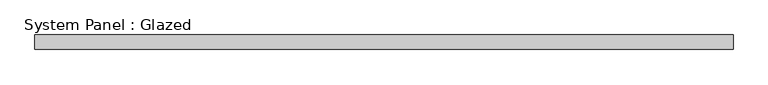
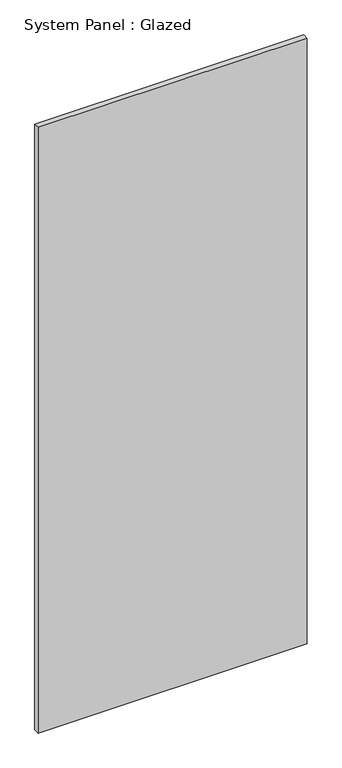
"""IFC4 building model written with IfcOpenShell, lengths in millimetres: plate geometry, System Panel : Glazed."""

from ifc_helpers import new_model, si_unit, origin, origin_with_axes, place, context, project, spatial, polyline, outline, extrude, source, transform, mapped, element, save


def system_panel_glazed_f99b9bb8(model_context):
    return source(origin(), model_context, "Body", "SweptSolid", [
        extrude(outline(polyline([(613.78773, 19.05), (-613.78773, 19.05), (-613.78773, 44.45), (613.78773, 44.45), (613.78773, 19.05)])), origin_with_axes(), (0.0, 0.0, 1.0), 2921.0),
    ])


if __name__ == "__main__":
    model = new_model("IFC4")
    model_context = context("Model", 3, world=origin())
    ifc_project = project(units=[si_unit("LENGTHUNIT", "METRE", prefix="MILLI")], contexts=[model_context])
    site = spatial("IfcSite", under=ifc_project)
    building = spatial("IfcBuilding", under=site)
    placement = place(None, origin())
    system_panel_glazed_shape = system_panel_glazed_f99b9bb8(model_context)
    element("IfcPlate", 1, ObjectType="System Panel : Glazed", at=placement, inside=building, context=model_context, shape_type="MappedRepresentation", body=[
        mapped(system_panel_glazed_shape, transform((0.0, 0.0, 0.0), x_axis=(1.0, 0.0, 0.0), y_axis=(0.0, 1.0, 0.0), z_axis=(0.0, 0.0, 1.0))),
    ])
    save(model, "model.ifc")

# Revit data of these elements
# Type "System Panel : Glazed"
#   Construction Type Id = "GSP4R"
#   Analytic Construction = "1/8 in Pilkington single glazing"
#   Visual Light Transmittance = 0.9
#   Solar Heat Gain Coefficient = 0.86
#   Heat Transfer Coefficient (U) = 1.18115 BTU/(h·ft²·°F)
# Element 1 (IfcPlate, "System Panel : Glazed")
#   Materials on its faces: "Glass"
# Materials
#   "Glass": class "Glass", colour RGB 0 128 192, transparency 0.75, Description = "Soda Lime Glass", Cost = 0
